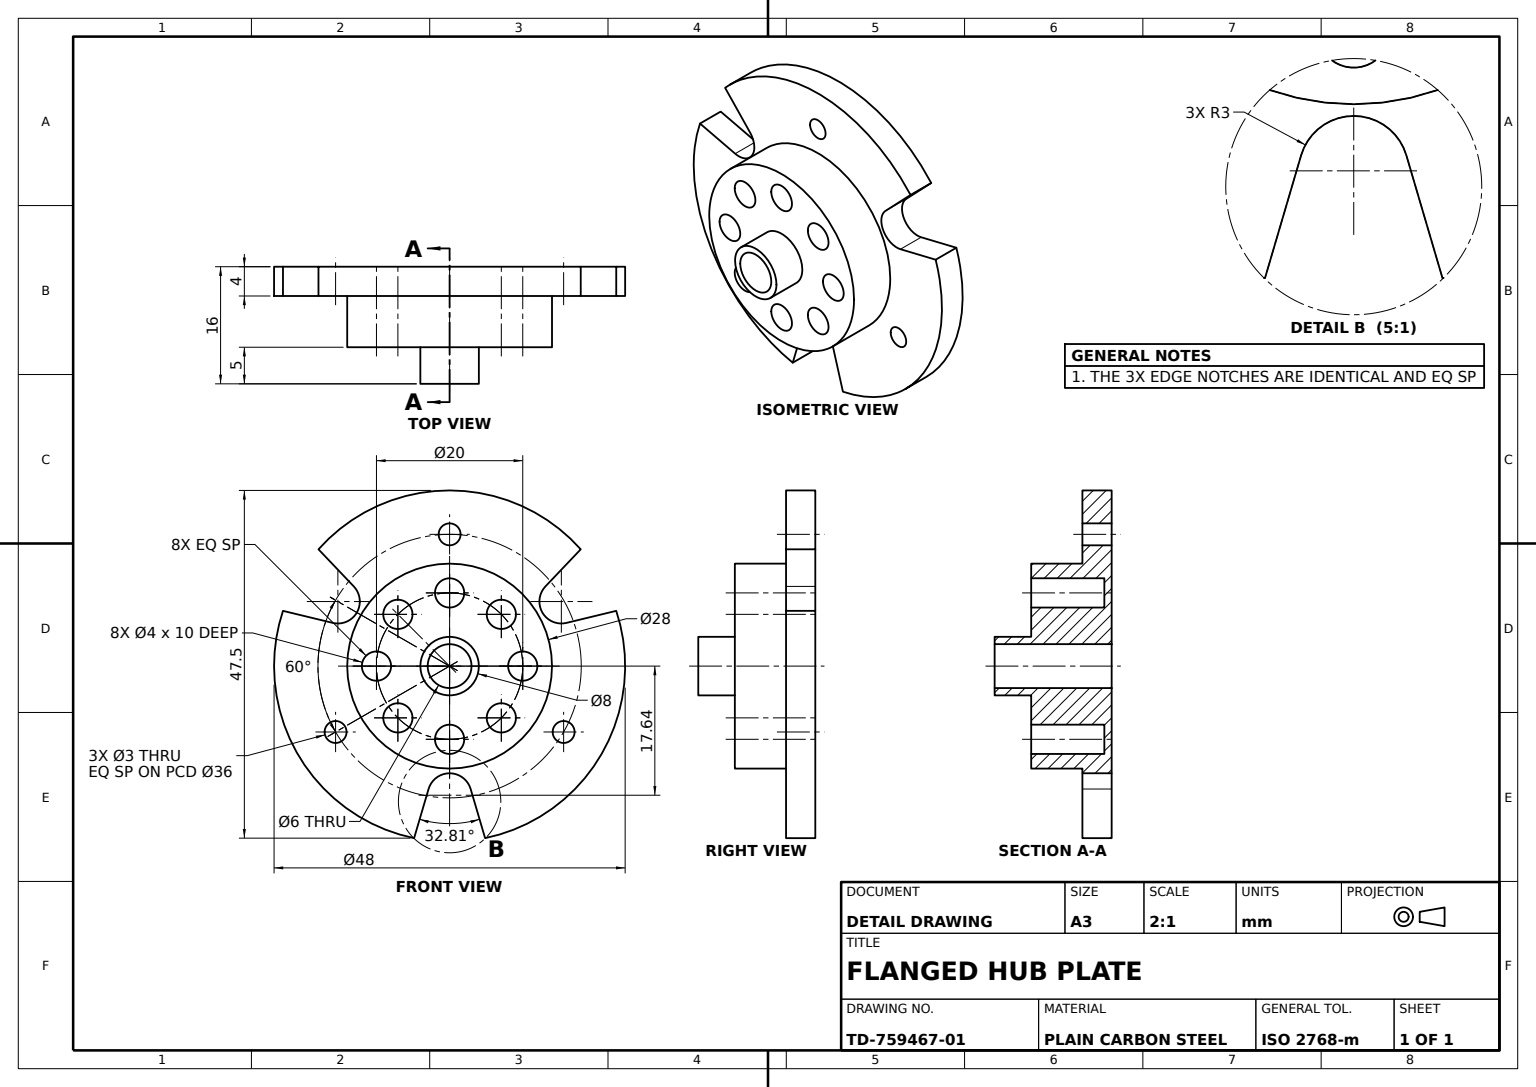
SolidWorks part; units mm, degrees
material "Plain Carbon Steel"
ref_plane "Front Plane" through (0, 0, 0) normal (0, 0, 1) x (1, 0, 0)
ref_plane "Top Plane" through (0, 0, 0) normal (0, 1, 0) x (1, 0, 0)
ref_plane "Right Plane" through (0, 0, 0) normal (1, 0, 0) x (0, 0, -1)
sketch "Flange Disc Sketch" plane through (0, 0, 0) normal (0, 0, 1) x (1, 0, 0)
  circle A0 centre (0, 0) radius 24
  dimension "D1" = 48
extrude "Flange Disc Ø48" add sketch "Flange Disc Sketch" along normal blind 4
sketch "Hub Sketch" plane through (0, 0, 4) normal (0, 0, 1) x (1, 0, 0)
  circle A0 centre (0, 0) radius 14
  dimension "D1" = 28
extrude "Hub Ø28" add sketch "Hub Sketch" along normal blind 7
sketch "Flange Holes Sketch" plane through (0, 0, 4) normal (0, 0, 1) x (1, 0, 0)
  circle A0 centre (0, 0) radius 18
  circle A1 centre (0, 18) radius 1.5
  circle A2 centre (15.5885, -9) radius 1.5
  circle A3 centre (-15.5885, -9) radius 1.5
  dimension "D1" = 36
  dimension "D2" = 3
  dimension "D4" = 9
  dimension "D5" = 15.5885
  dimension "D3" = 3
extrude "Flange Holes 3xØ3" cut sketch "Flange Holes Sketch" against normal blind 10 contours A0 A3 | A0 A3 | A0 A2 | A0 A2 | A0 A1 | A0 A1
sketch "Hub Holes Sketch" plane through (0, 0, 11) normal (0, 0, 1) x (1, 0, 0)
  circle A0 centre (0, 0) radius 10
  circle A1 centre (0, 10) radius 2
  circle A2 centre (7.0711, 7.0711) radius 2
  circle A3 centre (10, 0) radius 2
  circle A4 centre (7.0711, -7.0711) radius 2
  circle A5 centre (0, -10) radius 2
  circle A6 centre (-7.0711, -7.0711) radius 2
  circle A7 centre (-10, 0) radius 2
  circle A8 centre (-7.0711, 7.0711) radius 2
  dimension "D1" = 20
  dimension "D2" = 4
  dimension "D5" = 7.0711
  dimension "D3" = 2.9289
  dimension "D4" = 8
extrude "Hub Holes 8xØ4" cut sketch "Hub Holes Sketch" against normal blind 10 contours A0 A1 | A0 A2 | A0 A2 | A0 A3 | A0 A8 | A0 A8 | A0 A7 | A0 A7 | A0 A4 | A0 A4 | A0 A5 | A0 A5 | A0 A6 | A0 A6
sketch "Centre Spigot Sketch" plane through (0, 0, 11) normal (0, 0, 1) x (1, 0, 0)
  circle A0 centre (0, 0) radius 4
  dimension "D1" = 8
extrude "Centre Spigot Ø8" add sketch "Centre Spigot Sketch" along normal blind 5
sketch "Bore Sketch" plane through (0, 0, 16) normal (0, 0, 1) x (1, 0, 0)
  circle A0 centre (0, 0) radius 3
  dimension "D1" = 6
extrude "Bore Ø6" cut sketch "Bore Sketch" against normal blind 30
sketch "Edge Notches Sketch" plane through (0, 0, 4) normal (0, 0, 1) x (1, 0, 0)
  line L1 (-4.854, -23.504) -> (-2.8778, -16.7926)
  line L3 (4.854, -23.504) -> (2.8778, -16.7926)
  line L4 (-22.7821, 7.5484) -> (-15.9818, 5.904)
  line L5 (17.9281, 15.9557) -> (13.1039, 10.8886)
  line L6 (-17.9281, 15.9557) -> (-13.1039, 10.8886)
  line L7 (22.7821, 7.5484) -> (15.9818, 5.904)
  circle A0 centre (0, 0) radius 17.64
  arc A1 (2.8778, -16.7926) -> (-2.8778, -16.7926) centre (0, -17.64) ccw
  arc A3 (-4.854, -23.504) -> (4.854, -23.504) centre (0, 0) ccw
  arc A4 (-15.9818, 5.904) -> (-13.1039, 10.8886) centre (-15.2767, 8.82) ccw
  arc A5 (13.1039, 10.8886) -> (15.9818, 5.904) centre (15.2767, 8.82) ccw
  arc A6 (-17.9281, 15.9557) -> (-22.7821, 7.5484) centre (0, 0) ccw
  arc A7 (22.7821, 7.5484) -> (17.9281, 15.9557) centre (0, 0) ccw
  circle M7 centre (0, 0) radius 24
  dimension "D1" = 35.28
  dimension "D2" = 3
  dimension "D5" = 7.5484
  dimension "D3" = 9.7079
  dimension "D4" = 5.864
extrude "Edge Notches" cut sketch "Edge Notches Sketch" against normal blind 30 contours A0 L6 L4 M7 | L4 A4 L6 A0 | A0 L7 L5 M7 | L5 A5 L7 A0 | A0 L1 L3 M7 | L3 A1 L1 A0
